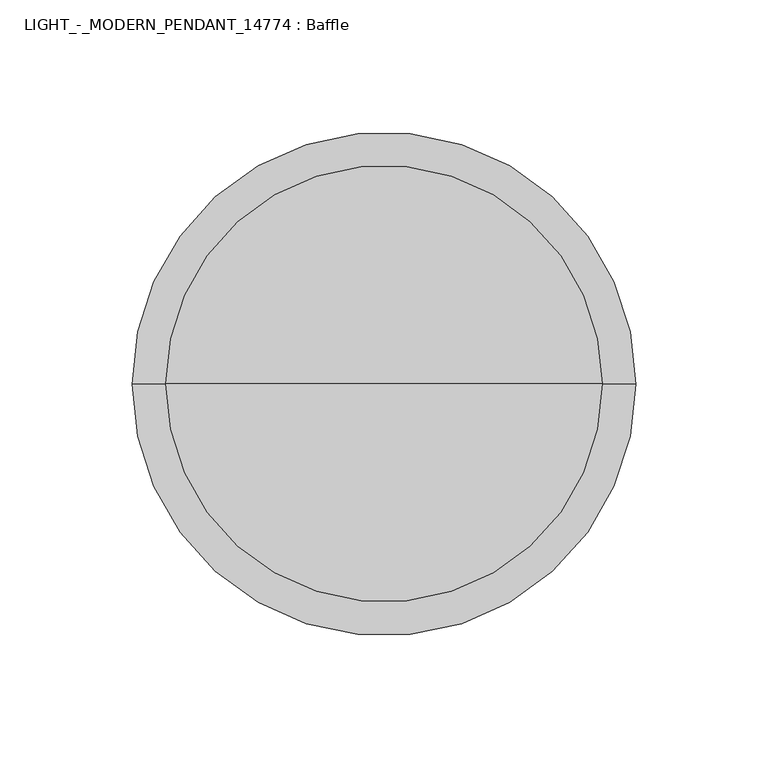
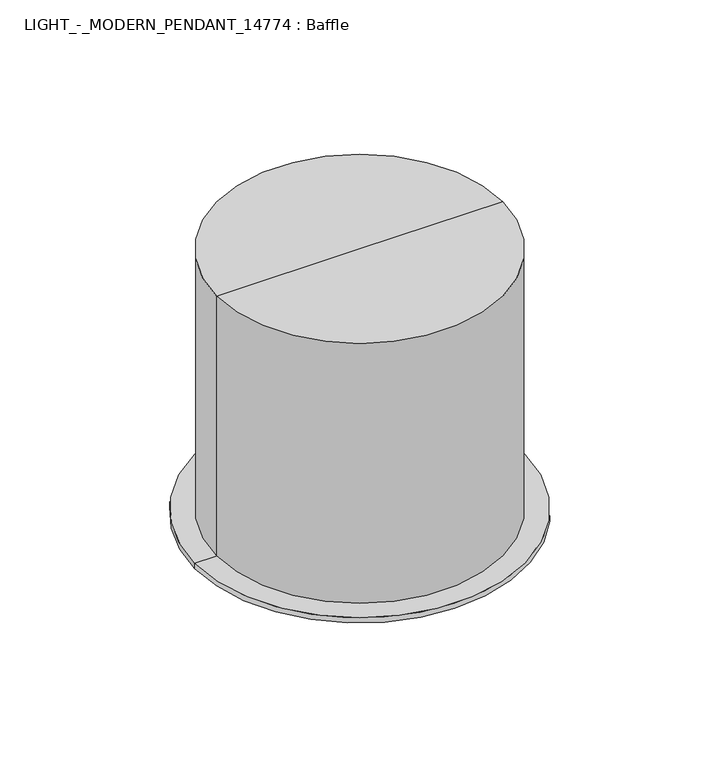
"""IFC4 building model written with IfcOpenShell, lengths in millimetres: light fixture geometry, LIGHT_-_MODERN_PENDANT_14774 : Baffle."""

from ifc_helpers import new_model, si_unit, frame, origin, place, context, project, spatial, polyline, circle_curve, source, transform, mapped, element, save
from ifc_brep_helpers import plane_surface, cylinder_surface, revolved_surface, advanced_brep


def light_modern_pendant_14774_baffle_b3430626(model_context):
    return source(origin(), model_context, "Body", "AdvancedBrep", [
        advanced_brep(
        [(-76.2, 0.0, 2438.4), (-76.2, 0.0, 2590.8), (76.2, 0.0, 2590.8), (76.2, 0.0, 2438.4), (-82.55, 0.0, 2438.4), (82.55, 0.0, 2438.4), (-82.55, 0.0, 2597.15), (82.55, 0.0, 2597.15), (0.0, 0.0, 2597.15), (0.0, 0.0, 2590.8)],
        [
            (0, 1),
            (1, 2, circle_curve(frame((0.0, 0.0, 2590.8), z_axis=(0.0, 0.0, 1.0), x_axis=(1.0, 0.0, 0.0)), 76.2)),
            (2, 3),
            (3, 0, circle_curve(frame((0.0, 0.0, 2438.4), z_axis=(0.0, 0.0, -1.0), x_axis=(1.0, 0.0, 0.0)), 76.2)),
            (2, 1, circle_curve(frame((0.0, 0.0, 2590.8), z_axis=(0.0, 0.0, 1.0), x_axis=(1.0, 0.0, 0.0)), 76.2)),
            (0, 3, circle_curve(frame((0.0, 0.0, 2438.4), z_axis=(0.0, 0.0, -1.0), x_axis=(1.0, 0.0, 0.0)), 76.2)),
            (4, 0),
            (3, 5),
            (5, 4, circle_curve(frame((0.0, 0.0, 2438.4), z_axis=(0.0, 0.0, -1.0), x_axis=(1.0, 0.0, 0.0)), 82.55)),
            (4, 5, circle_curve(frame((0.0, 0.0, 2438.4), z_axis=(0.0, 0.0, -1.0), x_axis=(1.0, 0.0, 0.0)), 82.55)),
            (6, 4),
            (5, 7),
            (7, 6, circle_curve(frame((0.0, 0.0, 2597.15), z_axis=(0.0, 0.0, -1.0), x_axis=(1.0, 0.0, 0.0)), 82.55)),
            (6, 7, circle_curve(frame((0.0, 0.0, 2597.15), z_axis=(0.0, 0.0, -1.0), x_axis=(1.0, 0.0, 0.0)), 82.55)),
            (8, 6),
            (7, 8),
            (1, 9),
            (9, 2),
        ],
        [
            revolved_surface(polyline([(76.2, 0.0, 2590.8), (76.2, 0.0, 2438.4)]), (0.0, 0.0, 2438.4), (0.0, 0.0, 1.0)),
            plane_surface(frame((0.0, 0.0, 2438.4), z_axis=(0.0, 0.0, -1.0), x_axis=(1.0, 0.0, 0.0))),
            cylinder_surface(frame((0.0, 0.0, 2438.4), z_axis=(0.0, 0.0, 1.0), x_axis=(1.0, 0.0, 0.0)), 82.55),
            plane_surface(frame((0.0, 0.0, 2597.15), z_axis=(0.0, 0.0, 1.0), x_axis=(1.0, 0.0, 0.0))),
            plane_surface(frame((0.0, 0.0, 2590.8), z_axis=(0.0, 0.0, -1.0), x_axis=(1.0, 0.0, 0.0))),
        ],
        [
            (0, [[1, 2, 3, 4]]),
            (0, [[-3, 5, -1, 6]]),
            (1, [[7, -4, 8, 9]]),
            (1, [[-8, -6, -7, 10]]),
            (2, [[11, -9, 12, 13]]),
            (2, [[-12, -10, -11, 14]]),
            (3, [[15, -13, 16]]),
            (3, [[-16, -14, -15]]),
            (4, [[17, 18, -2]]),
            (4, [[-18, -17, -5]]),
        ],
    ),
        advanced_brep(
        [(76.2, 0.0, 2473.3352136), (66.6647864, 0.0, 2463.8), (-66.6647864, 0.0, 2463.8), (-76.2, 0.0, 2473.3352136), (76.2, 0.0, 2438.4), (-76.2, 0.0, 2438.4), (71.3980217, 0.0, 2438.4), (-71.3980217, 0.0, 2438.4), (71.3980217, 0.0, 2444.75), (-71.3980217, 0.0, 2444.75), (69.8397864, 0.0, 2444.75), (-69.8397864, 0.0, 2444.75), (69.8397864, 0.0, 2451.1), (-69.8397864, 0.0, 2451.1), (68.2522864, 0.0, 2451.1), (-68.2522864, 0.0, 2451.1), (68.2522864, 0.0, 2457.45), (-68.2522864, 0.0, 2457.45), (66.6647864, 0.0, 2457.45), (-66.6647864, 0.0, 2457.45)],
        [
            (0, 1),
            (1, 2, circle_curve(frame((0.0, 0.0, 2463.8), z_axis=(0.0, 0.0, -1.0), x_axis=(-1.0, 0.0, 0.0)), 66.6647864)),
            (2, 3),
            (3, 0, circle_curve(frame((0.0, 0.0, 2473.3352136), z_axis=(0.0, 0.0, 1.0), x_axis=(-1.0, 0.0, 0.0)), 76.2)),
            (2, 1, circle_curve(frame((0.0, 0.0, 2463.8), z_axis=(0.0, 0.0, -1.0), x_axis=(-1.0, 0.0, 0.0)), 66.6647864)),
            (0, 3, circle_curve(frame((0.0, 0.0, 2473.3352136), z_axis=(0.0, 0.0, 1.0), x_axis=(-1.0, 0.0, 0.0)), 76.2)),
            (4, 0),
            (3, 5),
            (5, 4, circle_curve(frame((0.0, 0.0, 2438.4), z_axis=(0.0, 0.0, 1.0), x_axis=(-1.0, 0.0, 0.0)), 76.2)),
            (4, 5, circle_curve(frame((0.0, 0.0, 2438.4), z_axis=(0.0, 0.0, 1.0), x_axis=(-1.0, 0.0, 0.0)), 76.2)),
            (6, 4),
            (5, 7),
            (7, 6, circle_curve(frame((0.0, 0.0, 2438.4), z_axis=(0.0, 0.0, 1.0), x_axis=(-1.0, 0.0, 0.0)), 71.3980217)),
            (6, 7, circle_curve(frame((0.0, 0.0, 2438.4), z_axis=(0.0, 0.0, 1.0), x_axis=(-1.0, 0.0, 0.0)), 71.3980217)),
            (8, 6),
            (7, 9),
            (9, 8, circle_curve(frame((0.0, 0.0, 2444.75), z_axis=(0.0, 0.0, 1.0), x_axis=(-1.0, 0.0, 0.0)), 71.3980217)),
            (8, 9, circle_curve(frame((0.0, 0.0, 2444.75), z_axis=(0.0, 0.0, 1.0), x_axis=(-1.0, 0.0, 0.0)), 71.3980217)),
            (10, 8),
            (9, 11),
            (11, 10, circle_curve(frame((0.0, 0.0, 2444.75), z_axis=(0.0, 0.0, 1.0), x_axis=(-1.0, 0.0, 0.0)), 69.8397864)),
            (10, 11, circle_curve(frame((0.0, 0.0, 2444.75), z_axis=(0.0, 0.0, 1.0), x_axis=(-1.0, 0.0, 0.0)), 69.8397864)),
            (12, 10),
            (11, 13),
            (13, 12, circle_curve(frame((0.0, 0.0, 2451.1), z_axis=(0.0, 0.0, 1.0), x_axis=(-1.0, 0.0, 0.0)), 69.8397864)),
            (12, 13, circle_curve(frame((0.0, 0.0, 2451.1), z_axis=(0.0, 0.0, 1.0), x_axis=(-1.0, 0.0, 0.0)), 69.8397864)),
            (14, 12),
            (13, 15),
            (15, 14, circle_curve(frame((0.0, 0.0, 2451.1), z_axis=(0.0, 0.0, 1.0), x_axis=(-1.0, 0.0, 0.0)), 68.2522864)),
            (14, 15, circle_curve(frame((0.0, 0.0, 2451.1), z_axis=(0.0, 0.0, 1.0), x_axis=(-1.0, 0.0, 0.0)), 68.2522864)),
            (16, 14),
            (15, 17),
            (17, 16, circle_curve(frame((0.0, 0.0, 2457.45), z_axis=(0.0, 0.0, 1.0), x_axis=(-1.0, 0.0, 0.0)), 68.2522864)),
            (16, 17, circle_curve(frame((0.0, 0.0, 2457.45), z_axis=(0.0, 0.0, 1.0), x_axis=(-1.0, 0.0, 0.0)), 68.2522864)),
            (18, 16),
            (17, 19),
            (19, 18, circle_curve(frame((0.0, 0.0, 2457.45), z_axis=(0.0, 0.0, 1.0), x_axis=(-1.0, 0.0, 0.0)), 66.6647864)),
            (18, 19, circle_curve(frame((0.0, 0.0, 2457.45), z_axis=(0.0, 0.0, 1.0), x_axis=(-1.0, 0.0, 0.0)), 66.6647864)),
            (1, 18),
            (19, 2),
        ],
        [
            revolved_surface(polyline([(-66.6647864, 0.0, 2463.8), (-76.2, 0.0, 2473.3352136)]), (0.0, 0.0, 2584.45), (0.0, 0.0, -1.0)),
            cylinder_surface(frame((0.0, 0.0, 2584.45), z_axis=(0.0, 0.0, -1.0), x_axis=(-1.0, 0.0, 0.0)), 76.2),
            plane_surface(frame((0.0, 0.0, 2438.4), z_axis=(0.0, 0.0, -1.0), x_axis=(-1.0, 0.0, 0.0))),
            revolved_surface(polyline([(-71.3980217, 0.0, 2438.4), (-71.3980217, 0.0, 2444.75)]), (0.0, 0.0, 2584.45), (0.0, 0.0, -1.0)),
            plane_surface(frame((0.0, 0.0, 2444.75), z_axis=(0.0, 0.0, -1.0), x_axis=(-1.0, 0.0, 0.0))),
            revolved_surface(polyline([(-69.8397864, 0.0, 2444.75), (-69.8397864, 0.0, 2451.1)]), (0.0, 0.0, 2584.45), (0.0, 0.0, -1.0)),
            plane_surface(frame((0.0, 0.0, 2451.1), z_axis=(0.0, 0.0, -1.0), x_axis=(-1.0, 0.0, 0.0))),
            revolved_surface(polyline([(-68.2522864, 0.0, 2451.1), (-68.2522864, 0.0, 2457.45)]), (0.0, 0.0, 2584.45), (0.0, 0.0, -1.0)),
            plane_surface(frame((0.0, 0.0, 2457.45), z_axis=(0.0, 0.0, -1.0), x_axis=(-1.0, 0.0, 0.0))),
            revolved_surface(polyline([(-66.6647864, 0.0, 2457.45), (-66.6647864, 0.0, 2463.8)]), (0.0, 0.0, 2584.45), (0.0, 0.0, -1.0)),
        ],
        [
            (0, [[1, 2, 3, 4]]),
            (0, [[-3, 5, -1, 6]]),
            (1, [[7, -4, 8, 9]]),
            (1, [[-8, -6, -7, 10]]),
            (2, [[11, -9, 12, 13]]),
            (2, [[-12, -10, -11, 14]]),
            (3, [[15, -13, 16, 17]]),
            (3, [[-16, -14, -15, 18]]),
            (4, [[19, -17, 20, 21]]),
            (4, [[-20, -18, -19, 22]]),
            (5, [[23, -21, 24, 25]]),
            (5, [[-24, -22, -23, 26]]),
            (6, [[27, -25, 28, 29]]),
            (6, [[-28, -26, -27, 30]]),
            (7, [[31, -29, 32, 33]]),
            (7, [[-32, -30, -31, 34]]),
            (8, [[35, -33, 36, 37]]),
            (8, [[-36, -34, -35, 38]]),
            (9, [[39, -37, 40, -2]]),
            (9, [[-40, -38, -39, -5]]),
        ],
    ),
        advanced_brep(
        [(73.0147864, 0.0, 2438.4), (73.0147864, 0.0, 2432.05), (-73.0147864, 0.0, 2432.05), (-73.0147864, 0.0, 2438.4), (95.25, 0.0, 2438.4), (-95.25, 0.0, 2438.4), (95.25, 0.0, 2435.1749555), (-95.25, 0.0, 2435.1749555), (76.2, 0.0, 2432.05), (-76.2, 0.0, 2432.05)],
        [
            (0, 1),
            (1, 2, circle_curve(frame((0.0, 0.0, 2432.05), z_axis=(0.0, 0.0, -1.0), x_axis=(-1.0, 0.0, 0.0)), 73.0147864)),
            (2, 3),
            (3, 0, circle_curve(frame((0.0, 0.0, 2438.4), z_axis=(0.0, 0.0, 1.0), x_axis=(-1.0, 0.0, 0.0)), 73.0147864)),
            (2, 1, circle_curve(frame((0.0, 0.0, 2432.05), z_axis=(0.0, 0.0, -1.0), x_axis=(-1.0, 0.0, 0.0)), 73.0147864)),
            (0, 3, circle_curve(frame((0.0, 0.0, 2438.4), z_axis=(0.0, 0.0, 1.0), x_axis=(-1.0, 0.0, 0.0)), 73.0147864)),
            (4, 0),
            (3, 5),
            (5, 4, circle_curve(frame((0.0, 0.0, 2438.4), z_axis=(0.0, 0.0, 1.0), x_axis=(-1.0, 0.0, 0.0)), 95.25)),
            (4, 5, circle_curve(frame((0.0, 0.0, 2438.4), z_axis=(0.0, 0.0, 1.0), x_axis=(-1.0, 0.0, 0.0)), 95.25)),
            (6, 4),
            (5, 7),
            (7, 6, circle_curve(frame((0.0, 0.0, 2435.1749555), z_axis=(0.0, 0.0, 1.0), x_axis=(-1.0, 0.0, 0.0)), 95.25)),
            (6, 7, circle_curve(frame((0.0, 0.0, 2435.1749555), z_axis=(0.0, 0.0, 1.0), x_axis=(-1.0, 0.0, 0.0)), 95.25)),
            (8, 6),
            (7, 9),
            (9, 8, circle_curve(frame((0.0, 0.0, 2432.05), z_axis=(0.0, 0.0, 1.0), x_axis=(-1.0, 0.0, 0.0)), 76.2)),
            (8, 9, circle_curve(frame((0.0, 0.0, 2432.05), z_axis=(0.0, 0.0, 1.0), x_axis=(-1.0, 0.0, 0.0)), 76.2)),
            (1, 8),
            (9, 2),
        ],
        [
            revolved_surface(polyline([(-73.0147864, 0.0, 2432.05), (-73.0147864, 0.0, 2438.4)]), (0.0, 0.0, 2584.45), (0.0, 0.0, -1.0)),
            plane_surface(frame((0.0, 0.0, 2438.4), z_axis=(0.0, 0.0, 1.0), x_axis=(-1.0, 0.0, 0.0))),
            cylinder_surface(frame((0.0, 0.0, 2584.45), z_axis=(0.0, 0.0, -1.0), x_axis=(-1.0, 0.0, 0.0)), 95.25),
            revolved_surface(polyline([(-95.25, 0.0, 2435.1749555), (-76.2, 0.0, 2432.05)]), (0.0, 0.0, 2584.45), (0.0, 0.0, -1.0)),
            plane_surface(frame((0.0, 0.0, 2432.05), z_axis=(0.0, 0.0, -1.0), x_axis=(-1.0, 0.0, 0.0))),
        ],
        [
            (0, [[1, 2, 3, 4]]),
            (0, [[-3, 5, -1, 6]]),
            (1, [[7, -4, 8, 9]]),
            (1, [[-8, -6, -7, 10]]),
            (2, [[11, -9, 12, 13]]),
            (2, [[-12, -10, -11, 14]]),
            (3, [[15, -13, 16, 17]]),
            (3, [[-16, -14, -15, 18]]),
            (4, [[19, -17, 20, -2]]),
            (4, [[-20, -18, -19, -5]]),
        ],
    ),
    ])


if __name__ == "__main__":
    model = new_model("IFC4")
    model_context = context("Model", 3, world=origin())
    ifc_project = project(units=[si_unit("LENGTHUNIT", "METRE", prefix="MILLI")], contexts=[model_context])
    site = spatial("IfcSite", under=ifc_project)
    building = spatial("IfcBuilding", under=site)
    placement = place(None, origin())
    light_modern_pendant_14774_baffle_shape = light_modern_pendant_14774_baffle_b3430626(model_context)
    element("IfcLightFixture", 1, ObjectType="LIGHT_-_MODERN_PENDANT_14774 : Baffle", at=placement, inside=building, context=model_context, shape_type="MappedRepresentation", body=[
        mapped(light_modern_pendant_14774_baffle_shape, transform((0.0, 0.0, 0.0), x_axis=(1.0, 0.0, 0.0), y_axis=(0.0, 1.0, 0.0), z_axis=(0.0, 0.0, 1.0))),
    ])
    save(model, "model.ifc")

# Revit data of these elements
# Type "LIGHT_-_MODERN_PENDANT_14774 : Baffle"
#   Assembly Code = "D5020220"
#   Lamp = "A-19"
#   Wattage Comments = "60"
#   Wattage = 7.27067 W
#   built-in parameter 1150110 = 1 (stored number, unit not read)
#   built-in parameter 1114217 = 1 (stored number, unit not read)
#   Tilt Angle = 60.00°
#   built-in parameter 1150109 = 1 (stored number, unit not read)
#   built-in parameter 1150113 = 1 (stored number, unit not read)
#   built-in parameter 1010507 = 1.5708 (stored number, unit not read)
#   built-in parameter 1010506 = 0.523599 (stored number, unit not read)
#   built-in parameter 1150105 = 3611.05 (stored number, unit not read)
#   built-in parameter 1150115 = 1 (stored number, unit not read)
#   Light Source Symbol Length = 10' - 0"
#   built-in parameter 1150112 = 1 (stored number, unit not read)
#   built-in parameter 1150114 = 1 (stored number, unit not read)
#   built-in parameter 1150107 = 3200 (stored number, unit not read)
#   built-in parameter 1150106 = 36.1105 (stored number, unit not read)
#   built-in parameter 1150104 = 13.8 (stored number, unit not read)
#   built-in parameter 1114218 = 1 (stored number, unit not read)
#   built-in parameter 1150133 = 10 (stored number, unit not read)
#   Depth = 0' - 8"
#   Diameter = 0' - 6"
#   Lumens = 1080 lm
#   Wall Washer = no
#   Wall Wash Trim = no
#   built-in parameter 1150134 = 3
#   Reflector Cone = no
#   built-in parameter 1150132 = 2
#   Fresnel Lens = no
#   Color Filter = 16777215
#   Baffle = yes
#   Wall Wash Reflector [instance default] = none
#   Reflector [instance default] = none
#   Light Trim = Metal - Paint Finish - Ivory,Glossy
#   Fresnel Material [instance default] = none
#   Dimming Lamp Color Temperature Shift = (empty or 0)
#   Default Elevation = 0
# Element 1 (IfcLightFixture, "LIGHT_-_MODERN_PENDANT_14774 : Baffle")
#   Materials on its faces: "Metal - Paint Finish - Ivory,Glossy"
# Materials
#   "Metal - Paint Finish - Ivory,Glossy": colour RGB 247 247 239, transparency 0
